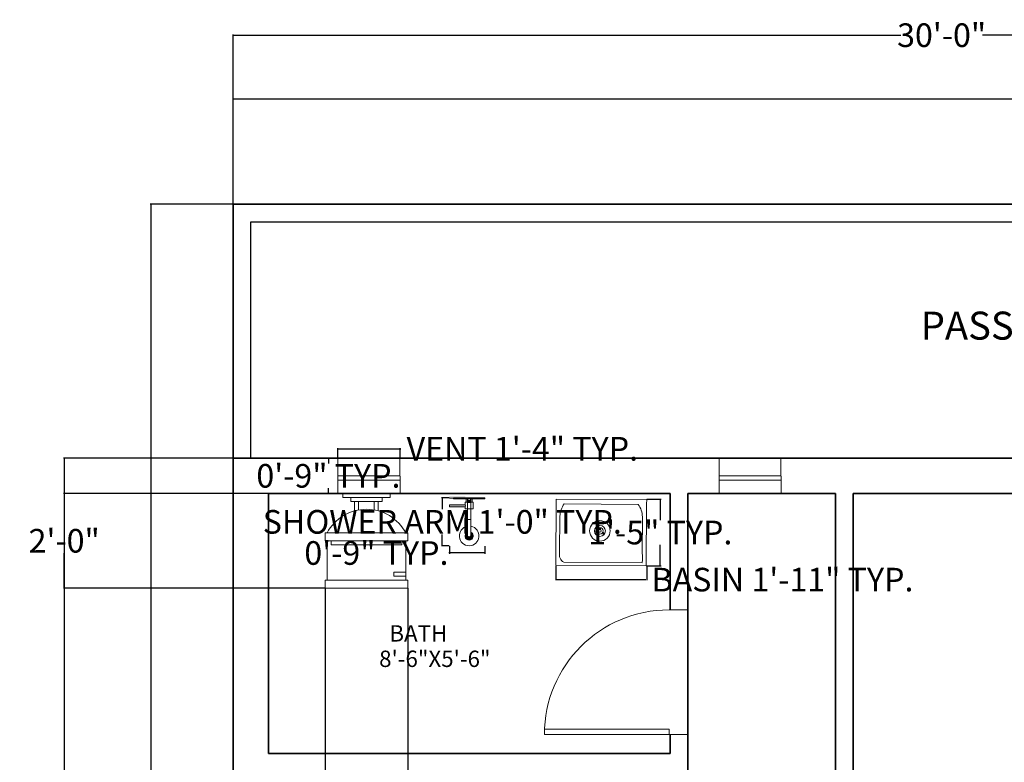
# Model space of a CAD drawing. Units: inches. Extents: x 79 to 8696167, y -3690578 to 147.
# Tile 5 of 10: x 79 to 329, y -42 to 147. Entities that reach past the tile are written whole.
import ezdxf

# ---------------------------------------------------------------- set-up
doc = ezdxf.new("R2010")
doc.units = ezdxf.units.IN
doc.header["$MEASUREMENT"] = 0
doc.layers.get('0').update_dxf_attribs({"color": 253})
for name, color, linetype, lineweight in [('A-ANNO-DIMS', 2, 'Continuous', 18), ('A-AREA-IDEN', 7, 'Continuous', 18), ('A-DOOR', 4, 'Continuous', 18), ('C-PROP', 7, 'Continuous', 35), ('C-SITE-WALL', 8, 'Continuous', 25), ('PLUMBING FIXTURES', 9, 'Continuous', 18), ('walls', 8, 'Continuous', 35), ('windows', 171, 'Continuous', 18)]:
    doc.layers.add(name, color=color, linetype=linetype, lineweight=lineweight)
doc.styles.get("Standard").update_dxf_attribs({"font": 'arial.ttf'})
doc.dimstyles.get("Standard").update_dxf_attribs({"dimtxt": 6, "dimasz": 0.18, "dimexe": 0.18, "dimexo": 0.0625, "dimgap": 0.09, "dimtad": 0, "dimtih": 1, "dimtoh": 1, "dimzin": 0, "dimdsep": 46, "dimlunit": 3, "dimtxsty": 'Standard', "dimcen": 0.09, "dimadec": 0, "dimazin": 0, "dimtfac": 1, "dimtofl": 0, "dimtmove": 0, "dimatfit": 3, "dimfxl": 1, "dimtolj": 1, "dimtzin": 0, "dimarcsym": 0})

# ---------------------------------------------------------------- blocks, each defined once
blk = doc.blocks.new('O.H SHOWER-PL')
at = {"layer": 'PLUMBING FIXTURES'}
for points in [[(-1.84, 0), (-1.84, -0.25), (1.84, -0.25), (1.84, 0)], [(0.46, -8.72), (0.46, -9.67, -0.422337), (-0.46, -9.67), (-0.46, -8.72, 4.325472)]]:
    blk.add_hatch(color=256, dxfattribs=at).paths.add_polyline_path(points)
for p, q in [((-1.84, 0), (-1.84, -0.25)), ((1.84, 0), (-1.84, 0)), ((1.84, 0), (1.84, -0.25)), ((1.84, -0.25), (-1.84, -0.25)), ((-0.46, -0.25), (-0.46, -9.67)), ((0.46, -0.25), (0.46, -9.67))]:
    blk.add_line(p, q, dxfattribs=at)
for centre, radius, start, end in [((0, -9.67), 2.5, 100.61, 79.39), ((0, -4.48), 1.03, 243.53, 296.47), ((0, -9.67), 1.05, 116.0349, 63.9652), ((0, -9.22), 0.643, 224.2078, 315.7922)]:
    blk.add_arc(centre, radius, start, end, dxfattribs=at)
blk = doc.blocks.new('DIVERTER-PL')
at = {"layer": 'PLUMBING FIXTURES'}
for points in [[(4, 0), (-4, 0), (-4, -0.25), (4, -0.25)], [(0.38, -1.14), (0.38, -0.7), (-0.37, -0.7), (-0.37, -1.14)], [(1, -1.75, 0.30818), (1, -2.25), (5, -2.25), (5, -1.75)]]:
    blk.add_hatch(color=256, dxfattribs=at).paths.add_polyline_path(points)
for p, q in [((-4, 0), (-4, -0.25)), ((-4, 0), (4, 0)), ((4, 0), (4, -0.25)), ((-4, -0.25), (4, -0.25)), ((-4, -0.25), (4, -0.25)), ((-1, -1.05), (-0.37, -1.05)), ((-1, -1.05), (-1, -2.75)), ((-0.75, -0.25), (-0.75, -1.05)), ((-0.37, -0.7), (0.38, -0.7)), ((-0.37, -0.7), (-0.37, -1.14)), ((-0.37, -1.14), (0.38, -1.14)), ((-0.32, -0.7), (-0.32, -0.25)), ((0.32, -0.7), (0.32, -0.25)), ((0.38, -0.7), (0.38, -1.14)), ((0.38, -1.05), (1, -1.05)), ((0.75, -0.25), (0.75, -1.05)), ((1, -1.05), (1, -1.75)), ((1, -2.25), (1, -2.75)), ((-1, -2.75), (1, -2.75))]:
    blk.add_line(p, q, dxfattribs=at)
at = {"layer": 'PLUMBING FIXTURES', "ltscale": 12}
for p, q in [((1, -1.75), (5, -1.75)), ((1, -2.25), (5, -2.25)), ((5, -2.25), (5, -1.75))]:
    blk.add_line(p, q, dxfattribs=at)
at = {"layer": 'PLUMBING FIXTURES'}
blk.add_arc((1.37, -2), 0.444, 145.7435, 214.2565, dxfattribs=at)
blk = doc.blocks.new('A$C7F153053')
at = {"layer": 'PLUMBING FIXTURES', "xscale": -1, "rotation": 270}
for name in ['DIVERTER-PL', 'O.H SHOWER-PL']:
    blk.add_blockref(name, (12.17, 4), dxfattribs=at)
blk = doc.blocks.new('*U10')
for p, q in [((-10, 22), (-10, 12)), ((-10, 21), (-7, 21)), ((-7, 21), (-7, 20)), ((10, 12), (10, 22)), ((-7, 20), (-10, 20)), ((9, 13), (-9, 13)), ((-9, 13), (-9, 12)), ((9, 12), (9, 13)), ((10.5, 12), (-10.5, 12)), ((-10.5, 10), (-10.5, 12)), ((10.5, 12), (10.5, 10)), ((10.5, 10), (-10.5, 10)), ((-3, 4.4065), (-3, 2)), ((-2, 2), (-2, 4.1658)), ((2, 4.1658), (2, 2)), ((3, 2), (3, 4.4065)), ((4, 2), (-4, 2)), ((-4, 2), (-4, 1)), ((4, 1), (4, 2))]:
    blk.add_line(p, q)
for points in [[(10.5, 22), (10.5, 24), (-10.5, 24), (-10.5, 22)], [(6, 0), (6, 1), (-6, 1), (-6, 0)]]:
    blk.add_lwpolyline(points, close=True)
blk.add_arc((0, 15.3333), 11.3333, 208.0725, 331.9275)
blk = doc.blocks.new('*U12')
for p, q in [((0, 0), (0, -6)), ((40, 0), (40, -6))]:
    blk.add_line(p, q)
blk.add_lwpolyline([(0, 0), (0, 40), (1.75, 40), (1.75, 0)], close=True)
blk.add_arc((0, 0), 40, 0, 90)
blk = doc.blocks.new('*D22')
at = {"layer": 'A-ANNO-DIMS', "color": 0, "lineweight": -2, "transparency": 16777216}
for p, q in [((133.44, 99.94), (133.44, 126.77)), ((133.62, 126.59), (338.26, 126.59)), ((553.26, 126.59), (348.62, 126.59)), ((553.44, 99.94), (553.44, 126.77))]:
    blk.add_line(p, q, dxfattribs=at)
at = {"layer": 'A-ANNO-DIMS', "color": 0, "lineweight": 100, "transparency": 16777216}
for points in [[(133.62, 126.62), (133.62, 126.56), (133.44, 126.59)], [(553.26, 126.62), (553.26, 126.56), (553.44, 126.59)]]:
    blk.add_solid(points, dxfattribs=at)
at = {"layer": 'Defpoints', "color": 0, "lineweight": 100, "transparency": 16777216}
for p in [(553.44, 126.59), (133.44, 99.88), (553.44, 99.88)]:
    blk.add_point(p, dxfattribs=at)
at = {"layer": 'A-ANNO-DIMS', "color": 0, "transparency": 16777216, "insert": (343.44, 126.59), "char_height": 6, "attachment_point": 5}
blk.add_mtext("\\A1;35'", dxfattribs=at)
blk = doc.blocks.new('*D23')
at = {"layer": 'A-ANNO-DIMS', "color": 0, "lineweight": -2, "transparency": 16777216}
for p, q in [((133.38, 99.88), (112.4, 99.88)), ((112.58, 99.7), (112.58, -286.97)), ((112.58, -679.94), (112.58, -293.28)), ((133.38, -680.12), (112.4, -680.12))]:
    blk.add_line(p, q, dxfattribs=at)
at = {"layer": 'A-ANNO-DIMS', "color": 0, "lineweight": 100, "transparency": 16777216}
for points in [[(112.55, 99.7), (112.61, 99.7), (112.58, 99.88)], [(112.55, -679.94), (112.61, -679.94), (112.58, -680.12)]]:
    blk.add_solid(points, dxfattribs=at)
at = {"layer": 'Defpoints', "color": 0, "lineweight": 100, "transparency": 16777216}
for p in [(112.58, 99.88), (133.44, 99.88), (133.44, -680.12)]:
    blk.add_point(p, dxfattribs=at)
at = {"layer": 'A-ANNO-DIMS', "color": 0, "transparency": 16777216, "insert": (112.58, -290.12), "char_height": 6, "attachment_point": 5}
blk.add_mtext("\\A1;65'", dxfattribs=at)
blk = doc.blocks.new('WIN-REAR-VENT')
for p, q in [((0, 0), (0, 9)), ((0, 9), (15.73, 9)), ((15.73, 9), (15.83, 0)), ((15.78, 4.5), (0, 4.5)), ((0, 0), (0, 3.42)), ((0, 3.42), (15.78, 3.42)), ((0.11, 0), (15.83, 0))]:
    blk.add_line(p, q)
blk = doc.blocks.new('BASIN-RECT-DRAIN')
for p, q in [((0, 0.15), (0.11, 17)), ((0.11, 17), (23.11, 16.85)), ((20.97, 15.65), (2.15, 15.77)), ((23.1, 15.71), (23, 0)), ((23.11, 16.85), (23.1, 15.71)), ((0.99, 3.35), (1.05, 12.64)), ((21.96, 3.21), (22.03, 12.5)), ((10.4, 8.91), (9.84, 8.81)), ((10.52, 8.7), (9.87, 8.58)), ((11.22, 9.73), (11.16, 9.24)), ((11.36, 9.22), (11.4, 9.7)), ((11.84, 8.39), (12.22, 7.95)), ((11.97, 8.6), (12.36, 8.13)), ((23, 0), (0, 0.15)), ((21.95, 0.84), (2.06, 0.97))]:
    blk.add_line(p, q)
for radius in [2.61, 1.39, 0.816, 0.338]:
    blk.add_circle((11.22, 8.91), radius)
for centre, radius, start, end in [((6.46, 12.5), 5.4, 142.7525, 178.5493), ((16.62, 12.43), 5.4, 0.6949, 36.4918), ((3, 2.82), 2.08, 165.2338, 242.9258), ((12.7, 2.09), 9.33, 352.3124, 6.9318)]:
    blk.add_arc(centre, radius, start, end)
blk = doc.blocks.new('SHOWER-HEAD-DETAIL')
for points in [[(4, 12.56, -0.30818), (4, 12.06), (0, 12.06), (0, 12.56)], [(4, 12.56, -0.30818), (4, 12.06), (0, 12.06), (0, 12.56)], [(4, 12.56, -0.30818), (4, 12.06), (0, 12.06), (0, 12.56)], [(4, 12.56, -0.30818), (4, 12.06), (0, 12.06), (0, 12.56)], [(4, 12.56, -0.30818), (4, 12.06), (0, 12.06), (0, 12.56)], [(4, 12.56, -0.30818), (4, 12.06), (0, 12.06), (0, 12.56)], [(4, 12.56, -0.30818), (4, 12.06), (0, 12.06), (0, 12.56)], [(4, 12.56, -0.30818), (4, 12.06), (0, 12.06), (0, 12.56)], [(4, 12.56, -0.30818), (4, 12.06), (0, 12.06), (0, 12.56)], [(4, 12.56, -0.30818), (4, 12.06), (0, 12.06), (0, 12.56)], [(4, 12.56, -0.30818), (4, 12.06), (0, 12.06), (0, 12.56)], [(4, 12.56, -0.30818), (4, 12.06), (0, 12.06), (0, 12.56)], [(4, 12.56, -0.30818), (4, 12.06), (0, 12.06), (0, 12.56)], [(4, 12.56, -0.30818), (4, 12.06), (0, 12.06), (0, 12.56)], [(4, 12.56, -0.30818), (4, 12.06), (0, 12.06), (0, 12.56)], [(4, 12.56, -0.30818), (4, 12.06), (0, 12.06), (0, 12.56)], [(4, 12.56, -0.30818), (4, 12.06), (0, 12.06), (0, 12.56)], [(4, 12.56, -0.30818), (4, 12.06), (0, 12.06), (0, 12.56)], [(4, 12.56, -0.30818), (4, 12.06), (0, 12.06), (0, 12.56)], [(4, 12.56, -0.30818), (4, 12.06), (0, 12.06), (0, 12.56)], [(4, 12.56, -0.30818), (4, 12.06), (0, 12.06), (0, 12.56)], [(4, 12.56, -0.30818), (4, 12.06), (0, 12.06), (0, 12.56)], [(4, 12.56, -0.30818), (4, 12.06), (0, 12.06), (0, 12.56)], [(4, 12.56, -0.30818), (4, 12.06), (0, 12.06), (0, 12.56)], [(4, 12.56, -0.30818), (4, 12.06), (0, 12.06), (0, 12.56)], [(4, 12.56, -0.30818), (4, 12.06), (0, 12.06), (0, 12.56)], [(4, 12.56, -0.30818), (4, 12.06), (0, 12.06), (0, 12.56)], [(4, 12.56, -0.30818), (4, 12.06), (0, 12.06), (0, 12.56)], [(4, 12.56, -0.30818), (4, 12.06), (0, 12.06), (0, 12.56)], [(4, 12.56, -0.30818), (4, 12.06), (0, 12.06), (0, 12.56)], [(4, 12.56, -0.30818), (4, 12.06), (0, 12.06), (0, 12.56)], [(4, 12.56, -0.30818), (4, 12.06), (0, 12.06), (0, 12.56)], [(4, 12.56, -0.30818), (4, 12.06), (0, 12.06), (0, 12.56)], [(4, 12.56, -0.30818), (4, 12.06), (0, 12.06), (0, 12.56)], [(4, 12.56, -0.30818), (4, 12.06), (0, 12.06), (0, 12.56)], [(4, 12.56, -0.30818), (4, 12.06), (0, 12.06), (0, 12.56)], [(4.54, 3.44), (4.54, 2.5, 0.422337), (5.46, 2.5), (5.46, 3.44, -4.325472)], [(4.54, 3.44), (4.54, 2.5, 0.422337), (5.46, 2.5), (5.46, 3.44, -4.325472)], [(4.54, 3.44), (4.54, 2.5, 0.422337), (5.46, 2.5), (5.46, 3.44, -4.325472)], [(4.54, 3.44), (4.54, 2.5, 0.422337), (5.46, 2.5), (5.46, 3.44, -4.325472)], [(4.54, 3.44), (4.54, 2.5, 0.422337), (5.46, 2.5), (5.46, 3.44, -4.325472)], [(4.54, 3.44), (4.54, 2.5, 0.422337), (5.46, 2.5), (5.46, 3.44, -4.325472)], [(4.54, 3.44), (4.54, 2.5, 0.422337), (5.46, 2.5), (5.46, 3.44, -4.325472)], [(4.54, 3.44), (4.54, 2.5, 0.422337), (5.46, 2.5), (5.46, 3.44, -4.325472)], [(4.54, 3.44), (4.54, 2.5, 0.422337), (5.46, 2.5), (5.46, 3.44, -4.325472)], [(4.54, 3.44), (4.54, 2.5, 0.422337), (5.46, 2.5), (5.46, 3.44, -4.325472)], [(4.54, 3.44), (4.54, 2.5, 0.422337), (5.46, 2.5), (5.46, 3.44, -4.325472)], [(4.54, 3.44), (4.54, 2.5, 0.422337), (5.46, 2.5), (5.46, 3.44, -4.325472)], [(4.54, 3.44), (4.54, 2.5, 0.422337), (5.46, 2.5), (5.46, 3.44, -4.325472)], [(4.54, 3.44), (4.54, 2.5, 0.422337), (5.46, 2.5), (5.46, 3.44, -4.325472)], [(4.54, 3.44), (4.54, 2.5, 0.422337), (5.46, 2.5), (5.46, 3.44, -4.325472)], [(4.54, 3.44), (4.54, 2.5, 0.422337), (5.46, 2.5), (5.46, 3.44, -4.325472)], [(4.54, 3.44), (4.54, 2.5, 0.422337), (5.46, 2.5), (5.46, 3.44, -4.325472)], [(4.54, 3.44), (4.54, 2.5, 0.422337), (5.46, 2.5), (5.46, 3.44, -4.325472)], [(4.54, 3.44), (4.54, 2.5, 0.422337), (5.46, 2.5), (5.46, 3.44, -4.325472)], [(4.54, 3.44), (4.54, 2.5, 0.422337), (5.46, 2.5), (5.46, 3.44, -4.325472)], [(4.54, 3.44), (4.54, 2.5, 0.422337), (5.46, 2.5), (5.46, 3.44, -4.325472)], [(4.54, 3.44), (4.54, 2.5, 0.422337), (5.46, 2.5), (5.46, 3.44, -4.325472)], [(4.54, 3.44), (4.54, 2.5, 0.422337), (5.46, 2.5), (5.46, 3.44, -4.325472)], [(4.54, 3.44), (4.54, 2.5, 0.422337), (5.46, 2.5), (5.46, 3.44, -4.325472)], [(4.54, 3.44), (4.54, 2.5, 0.422337), (5.46, 2.5), (5.46, 3.44, -4.325472)], [(4.54, 3.44), (4.54, 2.5, 0.422337), (5.46, 2.5), (5.46, 3.44, -4.325472)], [(4.54, 3.44), (4.54, 2.5, 0.422337), (5.46, 2.5), (5.46, 3.44, -4.325472)], [(4.54, 3.44), (4.54, 2.5, 0.422337), (5.46, 2.5), (5.46, 3.44, -4.325472)], [(4.54, 3.44), (4.54, 2.5, 0.422337), (5.46, 2.5), (5.46, 3.44, -4.325472)], [(4.54, 3.44), (4.54, 2.5, 0.422337), (5.46, 2.5), (5.46, 3.44, -4.325472)], [(4.54, 3.44), (4.54, 2.5, 0.422337), (5.46, 2.5), (5.46, 3.44, -4.325472)], [(4.54, 3.44), (4.54, 2.5, 0.422337), (5.46, 2.5), (5.46, 3.44, -4.325472)], [(4.54, 3.44), (4.54, 2.5, 0.422337), (5.46, 2.5), (5.46, 3.44, -4.325472)], [(4.54, 3.44), (4.54, 2.5, 0.422337), (5.46, 2.5), (5.46, 3.44, -4.325472)], [(4.54, 3.44), (4.54, 2.5, 0.422337), (5.46, 2.5), (5.46, 3.44, -4.325472)], [(4.54, 3.44), (4.54, 2.5, 0.422337), (5.46, 2.5), (5.46, 3.44, -4.325472)], [(4.54, 3.44), (4.54, 2.5, 0.422337), (5.46, 2.5), (5.46, 3.44, -4.325472)], [(4.54, 3.44), (4.54, 2.5, 0.422337), (5.46, 2.5), (5.46, 3.44, -4.325472)]]:
    blk.add_hatch(color=256).paths.add_polyline_path(points)
at = {"ltscale": 12}
blk.add_line((4, 12.06), (0, 12.06), dxfattribs=at)
blk.add_line((4, 12.06), (0, 12.06), dxfattribs=at)
blk.add_line((4, 12.06), (0, 12.06), dxfattribs=at)
blk.add_line((4, 12.06), (0, 12.06), dxfattribs=at)
blk.add_line((4, 12.06), (0, 12.06), dxfattribs=at)
blk.add_line((4, 12.06), (0, 12.06), dxfattribs=at)
blk.add_line((4, 12.06), (0, 12.06), dxfattribs=at)
blk.add_line((4, 12.06), (0, 12.06), dxfattribs=at)
blk.add_line((4, 12.06), (0, 12.06), dxfattribs=at)
blk.add_line((4, 12.06), (0, 12.06), dxfattribs=at)
blk.add_line((4, 12.06), (0, 12.06), dxfattribs=at)
blk.add_line((4, 12.06), (0, 12.06), dxfattribs=at)
blk.add_line((4, 12.06), (0, 12.06), dxfattribs=at)
blk.add_line((4, 12.06), (0, 12.06), dxfattribs=at)
blk.add_line((4, 12.06), (0, 12.06), dxfattribs=at)
blk.add_line((4, 12.06), (0, 12.06), dxfattribs=at)
blk.add_line((4, 12.06), (0, 12.06), dxfattribs=at)
blk.add_line((4, 12.06), (0, 12.06), dxfattribs=at)
blk.add_line((4, 12.06), (0, 12.06), dxfattribs=at)
blk.add_line((4, 12.06), (0, 12.06), dxfattribs=at)
blk.add_line((4, 12.06), (0, 12.06), dxfattribs=at)
blk.add_line((4, 12.06), (0, 12.06), dxfattribs=at)
blk.add_line((4, 12.06), (0, 12.06), dxfattribs=at)
blk.add_line((4, 12.06), (0, 12.06), dxfattribs=at)
blk.add_line((4, 12.06), (0, 12.06), dxfattribs=at)
blk.add_line((4, 12.06), (0, 12.06), dxfattribs=at)
blk.add_line((4, 12.06), (0, 12.06), dxfattribs=at)
blk.add_line((4, 12.06), (0, 12.06), dxfattribs=at)
blk.add_line((4, 12.06), (0, 12.06), dxfattribs=at)
blk.add_line((4, 12.06), (0, 12.06), dxfattribs=at)
blk.add_line((4, 12.06), (0, 12.06), dxfattribs=at)
blk.add_line((4, 12.06), (0, 12.06), dxfattribs=at)
blk.add_line((4, 12.06), (0, 12.06), dxfattribs=at)
blk.add_line((4, 12.06), (0, 12.06), dxfattribs=at)
blk.add_line((4, 12.06), (0, 12.06), dxfattribs=at)
blk.add_line((4, 12.06), (0, 12.06), dxfattribs=at)
blk.add_line((4, 12.06), (0, 12.06), dxfattribs=at)
blk.add_line((4, 12.06), (0, 12.06), dxfattribs=at)
for p, q in [((4.54, 11.92), (4.54, 2.5)), ((4.54, 11.92), (4.54, 2.5)), ((4.54, 11.92), (4.54, 2.5)), ((4.54, 11.92), (4.54, 2.5)), ((4.54, 11.92), (4.54, 2.5)), ((4.54, 11.92), (4.54, 2.5)), ((4.54, 11.92), (4.54, 2.5)), ((4.54, 11.92), (4.54, 2.5)), ((4.54, 11.92), (4.54, 2.5)), ((4.54, 11.92), (4.54, 2.5)), ((4.54, 11.92), (4.54, 2.5)), ((4.54, 11.92), (4.54, 2.5)), ((4.54, 11.92), (4.54, 2.5)), ((4.54, 11.92), (4.54, 2.5)), ((4.54, 11.92), (4.54, 2.5)), ((4.54, 11.92), (4.54, 2.5)), ((4.54, 11.92), (4.54, 2.5)), ((4.54, 11.92), (4.54, 2.5)), ((4.54, 11.92), (4.54, 2.5)), ((4.54, 11.92), (4.54, 2.5)), ((4.54, 11.92), (4.54, 2.5)), ((4.54, 11.92), (4.54, 2.5)), ((4.54, 11.92), (4.54, 2.5)), ((4.54, 11.92), (4.54, 2.5)), ((4.54, 11.92), (4.54, 2.5)), ((4.54, 11.92), (4.54, 2.5)), ((4.54, 11.92), (4.54, 2.5)), ((4.54, 11.92), (4.54, 2.5)), ((4.54, 11.92), (4.54, 2.5)), ((4.54, 11.92), (4.54, 2.5)), ((4.54, 11.92), (4.54, 2.5)), ((4.54, 11.92), (4.54, 2.5)), ((4.54, 11.92), (4.54, 2.5)), ((4.54, 11.92), (4.54, 2.5)), ((4.54, 11.92), (4.54, 2.5)), ((4.54, 11.92), (4.54, 2.5)), ((4.54, 11.92), (4.54, 2.5)), ((4.54, 11.92), (4.54, 2.5)), ((5.46, 11.92), (5.46, 2.5)), ((5.46, 11.92), (5.46, 2.5)), ((5.46, 11.92), (5.46, 2.5)), ((5.46, 11.92), (5.46, 2.5)), ((5.46, 11.92), (5.46, 2.5)), ((5.46, 11.92), (5.46, 2.5)), ((5.46, 11.92), (5.46, 2.5)), ((5.46, 11.92), (5.46, 2.5)), ((5.46, 11.92), (5.46, 2.5)), ((5.46, 11.92), (5.46, 2.5)), ((5.46, 11.92), (5.46, 2.5)), ((5.46, 11.92), (5.46, 2.5)), ((5.46, 11.92), (5.46, 2.5)), ((5.46, 11.92), (5.46, 2.5)), ((5.46, 11.92), (5.46, 2.5)), ((5.46, 11.92), (5.46, 2.5)), ((5.46, 11.92), (5.46, 2.5)), ((5.46, 11.92), (5.46, 2.5)), ((5.46, 11.92), (5.46, 2.5)), ((5.46, 11.92), (5.46, 2.5)), ((5.46, 11.92), (5.46, 2.5)), ((5.46, 11.92), (5.46, 2.5)), ((5.46, 11.92), (5.46, 2.5)), ((5.46, 11.92), (5.46, 2.5)), ((5.46, 11.92), (5.46, 2.5)), ((5.46, 11.92), (5.46, 2.5)), ((5.46, 11.92), (5.46, 2.5)), ((5.46, 11.92), (5.46, 2.5)), ((5.46, 11.92), (5.46, 2.5)), ((5.46, 11.92), (5.46, 2.5)), ((5.46, 11.92), (5.46, 2.5)), ((5.46, 11.92), (5.46, 2.5)), ((5.46, 11.92), (5.46, 2.5)), ((5.46, 11.92), (5.46, 2.5)), ((5.46, 11.92), (5.46, 2.5)), ((5.46, 11.92), (5.46, 2.5)), ((5.46, 11.92), (5.46, 2.5)), ((5.46, 11.92), (5.46, 2.5))]:
    blk.add_line(p, q)
for centre, radius, start, end in [((5, 7.69), 1.03, 243.53, 296.47), ((5, 7.69), 1.03, 243.53, 296.47), ((5, 7.69), 1.03, 243.53, 296.47), ((5, 7.69), 1.03, 243.53, 296.47), ((5, 7.69), 1.03, 243.53, 296.47), ((5, 7.69), 1.03, 243.53, 296.47), ((5, 7.69), 1.03, 243.53, 296.47), ((5, 7.69), 1.03, 243.53, 296.47), ((5, 7.69), 1.03, 243.53, 296.47), ((5, 7.69), 1.03, 243.53, 296.47), ((5, 7.69), 1.03, 243.53, 296.47), ((5, 7.69), 1.03, 243.53, 296.47), ((5, 7.69), 1.03, 243.53, 296.47), ((5, 7.69), 1.03, 243.53, 296.47), ((5, 7.69), 1.03, 243.53, 296.47), ((5, 7.69), 1.03, 243.53, 296.47), ((5, 7.69), 1.03, 243.53, 296.47), ((5, 7.69), 1.03, 243.53, 296.47), ((5, 7.69), 1.03, 243.53, 296.47), ((5, 7.69), 1.03, 243.53, 296.47), ((5, 7.69), 1.03, 243.53, 296.47), ((5, 7.69), 1.03, 243.53, 296.47), ((5, 7.69), 1.03, 243.53, 296.47), ((5, 7.69), 1.03, 243.53, 296.47), ((5, 7.69), 1.03, 243.53, 296.47), ((5, 7.69), 1.03, 243.53, 296.47), ((5, 7.69), 1.03, 243.53, 296.47), ((5, 7.69), 1.03, 243.53, 296.47), ((5, 7.69), 1.03, 243.53, 296.47), ((5, 7.69), 1.03, 243.53, 296.47), ((5, 7.69), 1.03, 243.53, 296.47), ((5, 7.69), 1.03, 243.53, 296.47), ((5, 7.69), 1.03, 243.53, 296.47), ((5, 7.69), 1.03, 243.53, 296.47), ((5, 7.69), 1.03, 243.53, 296.47), ((5, 7.69), 1.03, 243.53, 296.47), ((5, 7.69), 1.03, 243.53, 296.47), ((5, 7.69), 1.03, 243.53, 296.47), ((5, 2.5), 2.5, 100.61, 79.39), ((5, 2.5), 2.5, 100.61, 79.39), ((5, 2.5), 2.5, 100.61, 79.39), ((5, 2.5), 2.5, 100.61, 79.39), ((5, 2.5), 2.5, 100.61, 79.39), ((5, 2.5), 2.5, 100.61, 79.39), ((5, 2.5), 2.5, 100.61, 79.39), ((5, 2.5), 2.5, 100.61, 79.39), ((5, 2.5), 2.5, 100.61, 79.39), ((5, 2.5), 2.5, 100.61, 79.39), ((5, 2.5), 2.5, 100.61, 79.39), ((5, 2.5), 2.5, 100.61, 79.39), ((5, 2.5), 2.5, 100.61, 79.39), ((5, 2.5), 2.5, 100.61, 79.39), ((5, 2.5), 2.5, 100.61, 79.39), ((5, 2.5), 2.5, 100.61, 79.39), ((5, 2.5), 2.5, 100.61, 79.39), ((5, 2.5), 2.5, 100.61, 79.39), ((5, 2.5), 2.5, 100.61, 79.39), ((5, 2.5), 2.5, 100.61, 79.39), ((5, 2.5), 2.5, 100.61, 79.39), ((5, 2.5), 2.5, 100.61, 79.39), ((5, 2.5), 2.5, 100.61, 79.39), ((5, 2.5), 2.5, 100.61, 79.39), ((5, 2.5), 2.5, 100.61, 79.39), ((5, 2.5), 2.5, 100.61, 79.39), ((5, 2.5), 2.5, 100.61, 79.39), ((5, 2.5), 2.5, 100.61, 79.39), ((5, 2.5), 2.5, 100.61, 79.39), ((5, 2.5), 2.5, 100.61, 79.39), ((5, 2.5), 2.5, 100.61, 79.39), ((5, 2.5), 2.5, 100.61, 79.39), ((5, 2.5), 2.5, 100.61, 79.39), ((5, 2.5), 2.5, 100.61, 79.39), ((5, 2.5), 2.5, 100.61, 79.39), ((5, 2.5), 2.5, 100.61, 79.39), ((5, 2.5), 2.5, 100.61, 79.39), ((5, 2.5), 2.5, 100.61, 79.39), ((5, 2.5), 1.05, 116.0348, 63.9651), ((5, 2.5), 1.05, 116.0348, 63.9651), ((5, 2.5), 1.05, 116.0348, 63.9651), ((5, 2.5), 1.05, 116.0348, 63.9651), ((5, 2.5), 1.05, 116.0348, 63.9651), ((5, 2.5), 1.05, 116.0348, 63.9651), ((5, 2.5), 1.05, 116.0348, 63.9651), ((5, 2.5), 1.05, 116.0348, 63.9651), ((5, 2.5), 1.05, 116.0348, 63.9651), ((5, 2.5), 1.05, 116.0348, 63.9651), ((5, 2.5), 1.05, 116.0348, 63.9651), ((5, 2.5), 1.05, 116.0348, 63.9651), ((5, 2.5), 1.05, 116.0348, 63.9651), ((5, 2.5), 1.05, 116.0348, 63.9651), ((5, 2.5), 1.05, 116.0348, 63.9651), ((5, 2.5), 1.05, 116.0348, 63.9651), ((5, 2.5), 1.05, 116.0348, 63.9651), ((5, 2.5), 1.05, 116.0348, 63.9651), ((5, 2.5), 1.05, 116.0348, 63.9651), ((5, 2.5), 1.05, 116.0348, 63.9651), ((5, 2.5), 1.05, 116.0348, 63.9651), ((5, 2.5), 1.05, 116.0348, 63.9651), ((5, 2.5), 1.05, 116.0348, 63.9651), ((5, 2.5), 1.05, 116.0348, 63.9651), ((5, 2.5), 1.05, 116.0348, 63.9651), ((5, 2.5), 1.05, 116.0348, 63.9651), ((5, 2.5), 1.05, 116.0348, 63.9651), ((5, 2.5), 1.05, 116.0348, 63.9651), ((5, 2.5), 1.05, 116.0348, 63.9651), ((5, 2.5), 1.05, 116.0348, 63.9651), ((5, 2.5), 1.05, 116.0348, 63.9651), ((5, 2.5), 1.05, 116.0348, 63.9651), ((5, 2.5), 1.05, 116.0348, 63.9651), ((5, 2.5), 1.05, 116.0348, 63.9651), ((5, 2.5), 1.05, 116.0348, 63.9651), ((5, 2.5), 1.05, 116.0348, 63.9651), ((5, 2.5), 1.05, 116.0348, 63.9651), ((5, 2.5), 1.05, 116.0348, 63.9651), ((5, 2.95), 0.643, 224.2078, 315.7922), ((5, 2.95), 0.643, 224.2078, 315.7922), ((5, 2.95), 0.643, 224.2078, 315.7922), ((5, 2.95), 0.643, 224.2078, 315.7922), ((5, 2.95), 0.643, 224.2078, 315.7922), ((5, 2.95), 0.643, 224.2078, 315.7922), ((5, 2.95), 0.643, 224.2078, 315.7922), ((5, 2.95), 0.643, 224.2078, 315.7922), ((5, 2.95), 0.643, 224.2078, 315.7922), ((5, 2.95), 0.643, 224.2078, 315.7922), ((5, 2.95), 0.643, 224.2078, 315.7922), ((5, 2.95), 0.643, 224.2078, 315.7922), ((5, 2.95), 0.643, 224.2078, 315.7922), ((5, 2.95), 0.643, 224.2078, 315.7922), ((5, 2.95), 0.643, 224.2078, 315.7922), ((5, 2.95), 0.643, 224.2078, 315.7922), ((5, 2.95), 0.643, 224.2078, 315.7922), ((5, 2.95), 0.643, 224.2078, 315.7922), ((5, 2.95), 0.643, 224.2078, 315.7922), ((5, 2.95), 0.643, 224.2078, 315.7922), ((5, 2.95), 0.643, 224.2078, 315.7922), ((5, 2.95), 0.643, 224.2078, 315.7922), ((5, 2.95), 0.643, 224.2078, 315.7922), ((5, 2.95), 0.643, 224.2078, 315.7922), ((5, 2.95), 0.643, 224.2078, 315.7922), ((5, 2.95), 0.643, 224.2078, 315.7922), ((5, 2.95), 0.643, 224.2078, 315.7922), ((5, 2.95), 0.643, 224.2078, 315.7922), ((5, 2.95), 0.643, 224.2078, 315.7922), ((5, 2.95), 0.643, 224.2078, 315.7922), ((5, 2.95), 0.643, 224.2078, 315.7922), ((5, 2.95), 0.643, 224.2078, 315.7922), ((5, 2.95), 0.643, 224.2078, 315.7922), ((5, 2.95), 0.643, 224.2078, 315.7922), ((5, 2.95), 0.643, 224.2078, 315.7922), ((5, 2.95), 0.643, 224.2078, 315.7922), ((5, 2.95), 0.643, 224.2078, 315.7922), ((5, 2.95), 0.643, 224.2078, 315.7922)]:
    blk.add_arc(centre, radius, start, end)
blk = doc.blocks.new('*D31')
at = {"layer": 'A-ANNO-DIMS', "color": 0, "lineweight": -2, "transparency": 16777216}
for p, q in [((160.03, 35.44), (160.03, 37.93)), ((160.21, 37.75), (175.69, 37.75)), ((175.87, 35.44), (175.87, 37.93)), ((175.87, 37.75), (176.05, 37.75))]:
    blk.add_line(p, q, dxfattribs=at)
at = {"layer": 'A-ANNO-DIMS', "color": 0, "lineweight": 100, "transparency": 16777216}
for points in [[(160.21, 37.78), (160.21, 37.72), (160.03, 37.75)], [(175.69, 37.78), (175.69, 37.72), (175.87, 37.75)]]:
    blk.add_solid(points, dxfattribs=at)
at = {"layer": 'Defpoints', "color": 0, "lineweight": 100, "transparency": 16777216}
for p in [(175.87, 37.75), (160.03, 35.38), (175.87, 35.38)]:
    blk.add_point(p, dxfattribs=at)
at = {"layer": 'A-ANNO-DIMS', "color": 0, "transparency": 16777216, "insert": (206.92, 37.75), "char_height": 6, "attachment_point": 5}
blk.add_mtext('\\A1;VENT 1\'-4" TYP.', dxfattribs=at)
blk = doc.blocks.new('*D32')
at = {"layer": 'A-ANNO-DIMS', "color": 0, "lineweight": -2, "transparency": 16777216}
for p, q in [((159.97, 35.38), (157.48, 35.38)), ((157.66, 35.2), (157.66, 34.03)), ((157.66, 26.56), (157.66, 27.72)), ((159.97, 26.38), (157.48, 26.38))]:
    blk.add_line(p, q, dxfattribs=at)
at = {"layer": 'A-ANNO-DIMS', "color": 0, "lineweight": 100, "transparency": 16777216}
for points in [[(157.63, 35.2), (157.69, 35.2), (157.66, 35.38)], [(157.63, 26.56), (157.69, 26.56), (157.66, 26.38)]]:
    blk.add_solid(points, dxfattribs=at)
at = {"layer": 'Defpoints', "color": 0, "lineweight": 100, "transparency": 16777216}
for p in [(157.66, 35.38), (160.03, 35.38), (160.03, 26.38)]:
    blk.add_point(p, dxfattribs=at)
at = {"layer": 'A-ANNO-DIMS', "color": 0, "transparency": 16777216, "insert": (157.66, 30.88), "char_height": 6, "attachment_point": 5}
blk.add_mtext('\\A1;0\'-9" TYP.', dxfattribs=at)
blk = doc.blocks.new('*D43')
at = {"layer": 'A-ANNO-DIMS', "color": 0, "lineweight": -2, "transparency": 16777216}
for p, q in [((188.35, 25.27), (186.4, 25.27)), ((186.58, 25.09), (186.58, 22.38)), ((186.58, 13.28), (186.58, 15.99)), ((188.35, 13.1), (186.4, 13.1))]:
    blk.add_line(p, q, dxfattribs=at)
at = {"layer": 'A-ANNO-DIMS', "color": 0, "lineweight": 100, "transparency": 16777216}
for points in [[(186.55, 25.09), (186.61, 25.09), (186.58, 25.27)], [(186.55, 13.28), (186.61, 13.28), (186.58, 13.1)]]:
    blk.add_solid(points, dxfattribs=at)
at = {"layer": 'Defpoints', "color": 0, "lineweight": 100, "transparency": 16777216}
for p in [(186.58, 25.27), (188.41, 25.27), (188.41, 13.1)]:
    blk.add_point(p, dxfattribs=at)
at = {"layer": 'A-ANNO-DIMS', "color": 0, "transparency": 16777216, "insert": (186.58, 19.19), "char_height": 6, "attachment_point": 5}
blk.add_mtext('\\A1;SHOWER ARM 1\'-0" TYP.', dxfattribs=at)
blk = doc.blocks.new('*D44')
at = {"layer": 'A-ANNO-DIMS', "color": 0, "lineweight": -2, "transparency": 16777216}
for p, q in [((188.41, 13.04), (188.41, 11.1)), ((197.41, 13.04), (197.41, 11.1)), ((188.41, 11.28), (188.23, 11.28)), ((197.23, 11.28), (188.59, 11.28))]:
    blk.add_line(p, q, dxfattribs=at)
at = {"layer": 'A-ANNO-DIMS', "color": 0, "lineweight": 100, "transparency": 16777216}
for points in [[(188.59, 11.31), (188.59, 11.25), (188.41, 11.28)], [(197.23, 11.31), (197.23, 11.25), (197.41, 11.28)]]:
    blk.add_solid(points, dxfattribs=at)
at = {"layer": 'Defpoints', "color": 0, "lineweight": 100, "transparency": 16777216}
for p in [(188.41, 13.1), (197.41, 13.1), (188.41, 11.28)]:
    blk.add_point(p, dxfattribs=at)
at = {"layer": 'A-ANNO-DIMS', "color": 0, "transparency": 16777216, "insert": (169.85, 11.28), "char_height": 6, "attachment_point": 5}
blk.add_mtext('\\A1;0\'-9" TYP.', dxfattribs=at)
blk = doc.blocks.new('*D47')
at = {"layer": 'A-ANNO-DIMS', "color": 0, "lineweight": -2, "transparency": 16777216}
for p, q in [((215.4, 7.92), (215.4, 4.34)), ((238.51, 7.92), (238.51, 4.34)), ((215.58, 4.52), (238.33, 4.52)), ((238.51, 4.52), (238.69, 4.52))]:
    blk.add_line(p, q, dxfattribs=at)
at = {"layer": 'A-ANNO-DIMS', "color": 0, "lineweight": 100, "transparency": 16777216}
for points in [[(215.58, 4.55), (215.58, 4.49), (215.4, 4.52)], [(238.33, 4.55), (238.33, 4.49), (238.51, 4.52)]]:
    blk.add_solid(points, dxfattribs=at)
at = {"layer": 'Defpoints', "color": 0, "lineweight": 100, "transparency": 16777216}
for p in [(215.4, 7.98), (238.51, 7.98), (238.51, 4.52)]:
    blk.add_point(p, dxfattribs=at)
at = {"layer": 'A-ANNO-DIMS', "color": 0, "transparency": 16777216, "insert": (273, 4.52), "char_height": 6, "attachment_point": 5}
blk.add_mtext('\\A1;BASIN 1\'-11" TYP.', dxfattribs=at)
blk = doc.blocks.new('*D48')
at = {"layer": 'A-ANNO-DIMS', "color": 0, "lineweight": -2, "transparency": 16777216}
for p, q in [((238.57, 24.98), (242.15, 24.98)), ((241.97, 24.8), (241.97, 19.64)), ((241.97, 8.16), (241.97, 13.33)), ((238.57, 7.98), (242.15, 7.98))]:
    blk.add_line(p, q, dxfattribs=at)
at = {"layer": 'A-ANNO-DIMS', "color": 0, "lineweight": 100, "transparency": 16777216}
for points in [[(241.94, 24.8), (242, 24.8), (241.97, 24.98)], [(241.94, 8.16), (242, 8.16), (241.97, 7.98)]]:
    blk.add_solid(points, dxfattribs=at)
at = {"layer": 'Defpoints', "color": 0, "lineweight": 100, "transparency": 16777216}
for p in [(238.51, 24.98), (241.97, 24.98), (238.51, 7.98)]:
    blk.add_point(p, dxfattribs=at)
at = {"layer": 'A-ANNO-DIMS', "color": 0, "transparency": 16777216, "insert": (241.97, 16.48), "char_height": 6, "attachment_point": 5}
blk.add_mtext('\\A1;1\'-5" TYP.', dxfattribs=at)
blk = doc.blocks.new('*D55')
at = {"layer": 'A-ANNO-DIMS', "color": 0, "lineweight": -2, "transparency": 16777216}
for p, q in [((133.44, 35.44), (133.44, 142.96)), ((133.62, 142.78), (303.05, 142.78)), ((493.26, 142.78), (323.83, 142.78)), ((493.44, 35.44), (493.44, 142.96))]:
    blk.add_line(p, q, dxfattribs=at)
at = {"layer": 'A-ANNO-DIMS', "color": 0, "lineweight": 100, "transparency": 16777216}
for points in [[(133.62, 142.81), (133.62, 142.75), (133.44, 142.78)], [(493.26, 142.81), (493.26, 142.75), (493.44, 142.78)]]:
    blk.add_solid(points, dxfattribs=at)
at = {"layer": 'Defpoints', "color": 0, "lineweight": 100, "transparency": 16777216}
for p in [(493.44, 142.78), (133.44, 35.38), (493.44, 35.38)]:
    blk.add_point(p, dxfattribs=at)
at = {"layer": 'A-ANNO-DIMS', "color": 0, "transparency": 16777216, "insert": (313.44, 142.78), "char_height": 6, "attachment_point": 5}
blk.add_mtext('\\A1;30\'-0"', dxfattribs=at)
blk = doc.blocks.new('*D56')
at = {"layer": 'A-ANNO-DIMS', "color": 0, "lineweight": -2, "transparency": 16777216}
for p, q in [((133.38, 35.38), (90.36, 35.38)), ((90.54, 35.2), (90.54, -253.97)), ((90.54, -549.44), (90.54, -260.28)), ((133.38, -549.62), (90.36, -549.62))]:
    blk.add_line(p, q, dxfattribs=at)
at = {"layer": 'A-ANNO-DIMS', "color": 0, "lineweight": 100, "transparency": 16777216}
for points in [[(90.51, 35.2), (90.57, 35.2), (90.54, 35.38)], [(90.51, -549.44), (90.57, -549.44), (90.54, -549.62)]]:
    blk.add_solid(points, dxfattribs=at)
at = {"layer": 'Defpoints', "color": 0, "lineweight": 100, "transparency": 16777216}
for p in [(90.54, 35.38), (133.44, 35.38), (133.44, -549.62)]:
    blk.add_point(p, dxfattribs=at)
at = {"layer": 'A-ANNO-DIMS', "color": 0, "transparency": 16777216, "insert": (90.54, -257.12), "char_height": 6, "attachment_point": 5}
blk.add_mtext('\\A1;48\'-9"', dxfattribs=at)
blk = doc.blocks.new('*D59')
at = {"layer": 'A-ANNO-DIMS', "color": 0, "lineweight": -2, "transparency": 16777216}
for p, q in [((156.82, 2.31), (156.82, -723.2)), ((177.82, 2.31), (177.82, -723.2)), ((157, -723.02), (159.53, -723.02)), ((177.64, -723.02), (175.1, -723.02))]:
    blk.add_line(p, q, dxfattribs=at)
at = {"layer": 'A-ANNO-DIMS', "color": 0, "lineweight": 100, "transparency": 16777216}
for points in [[(157, -722.99), (157, -723.05), (156.82, -723.02)], [(177.64, -722.99), (177.64, -723.05), (177.82, -723.02)]]:
    blk.add_solid(points, dxfattribs=at)
at = {"layer": 'Defpoints', "color": 0, "lineweight": 100, "transparency": 16777216}
for p in [(156.82, 2.38), (177.82, 2.38), (177.82, -723.02)]:
    blk.add_point(p, dxfattribs=at)
at = {"layer": 'A-ANNO-DIMS', "color": 0, "transparency": 16777216, "insert": (167.32, -723.02), "char_height": 6, "attachment_point": 5}
blk.add_mtext('\\A1;1\'-9"', dxfattribs=at)
blk = doc.blocks.new('*D60')
at = {"layer": 'A-ANNO-DIMS', "color": 0, "lineweight": -2, "transparency": 16777216}
for p, q in [((161.25, 26.38), (90.36, 26.38)), ((90.54, 26.2), (90.54, 17.53)), ((90.54, 2.56), (90.54, 11.22)), ((156.75, 2.38), (90.36, 2.38))]:
    blk.add_line(p, q, dxfattribs=at)
at = {"layer": 'A-ANNO-DIMS', "color": 0, "lineweight": 100, "transparency": 16777216}
for points in [[(90.51, 26.2), (90.57, 26.2), (90.54, 26.38)], [(90.51, 2.56), (90.57, 2.56), (90.54, 2.38)]]:
    blk.add_solid(points, dxfattribs=at)
at = {"layer": 'Defpoints', "color": 0, "lineweight": 100, "transparency": 16777216}
for p in [(90.54, 26.38), (161.32, 26.38), (156.82, 2.38)]:
    blk.add_point(p, dxfattribs=at)
at = {"layer": 'A-ANNO-DIMS', "color": 0, "transparency": 16777216, "insert": (90.54, 14.38), "char_height": 6, "attachment_point": 5}
blk.add_mtext('\\A1;2\'-0"', dxfattribs=at)

msp = doc.modelspace()

# ---------------------------------------------------------------- linework, layer by layer
at = {"layer": 'C-PROP'}
for p, q in [((133.441, 99.875), (553.441, 99.875)), ((133.441, -680.125), (133.441, 99.875))]:
    msp.add_line(p, q, dxfattribs=at)
at = {"layer": 'C-SITE-WALL'}
for p, q in [((137.941, 95.375), (548.941, 95.375)), ((137.941, 35.375), (137.941, 95.375)), ((133.441, 35.375), (137.941, 35.375))]:
    msp.add_line(p, q, dxfattribs=at)
at = {"layer": 'walls'}
for p, q in [((133.441, 35.375), (493.441, 35.375)), ((142.441, 26.375), (244.441, 26.375)), ((142.441, -39.625), (142.441, 26.375)), ((244.441, -3.166), (244.441, 26.375)), ((248.941, -44.125), (248.941, 26.375)), ((248.941, 26.375), (286.441, 26.375)), ((286.441, -62.986), (286.441, 26.375)), ((290.941, -58.486), (290.941, 26.375)), ((290.941, 26.375), (484.441, 26.375)), ((244.441, -39.625), (244.441, -34.834)), ((142.441, -39.625), (244.441, -39.625))]:
    msp.add_line(p, q, dxfattribs=at)

# ---------------------------------------------------------------- block references
at = {"layer": 'A-DOOR', "xscale": 0.7916830879858355, "yscale": 0.7916830879858355, "zscale": 0.7916830879858355, "rotation": 90}
msp.add_blockref('*U12', (244.191, -34.834), dxfattribs=at)
at = {"layer": 'PLUMBING FIXTURES', "rotation": 180}
msp.add_blockref('*U10', (167.317, 26.375), dxfattribs=at)
at = {"layer": 'PLUMBING FIXTURES'}
for name, p in [('SHOWER-HEAD-DETAIL', (188.409, 13.104)), ('BASIN-RECT-DRAIN', (215.402, 7.982))]:
    msp.add_blockref(name, p, dxfattribs=at)
at = {"layer": 'PLUMBING FIXTURES', "ltscale": 35, "rotation": 89.99999999999999}
msp.add_blockref('A$C7F153053', (197.409, 13.106), dxfattribs=at)
at = {"layer": 'windows'}
for p in [(160.032, 26.375), (256.888, 26.375)]:
    msp.add_blockref('WIN-REAR-VENT', p, dxfattribs=at)

# ---------------------------------------------------------------- texts
at = {"layer": 'A-AREA-IDEN'}
for s, height, p in [('PASSAGE 5\'-4.5" WIDE', 7.11297, (308.132, 65.462)), ('BATH', 4.1556, (173.146, -11.214)), ('8\'-6"X5\'-6"', 4.15558, (170.546, -17.671))]:
    msp.add_text(s, height=height, dxfattribs=at).set_placement(p)

# ---------------------------------------------------------------- dimensions: what is measured, and where the dimension line sits
at = {"layer": 'A-ANNO-DIMS'}
for base, p1, p2, override, picture, middle in [((493.441, 142.775), (133.441, 35.375), (493.441, 35.375), {"dimdec": 1, "dimlfac": 1, "dimrnd": 0, "dimzin": 1, "dimdsep": 46, "dimlunit": 4, "dimfrac": 2}, '*D55', (313.441, 142.775)), ((553.441, 126.587), (133.441, 99.875), (553.441, 99.875), {"dimclrd": 0, "dimclre": 0, "dimclrt": 0}, '*D22', (343.441, 126.587)), ((177.817, -723.025), (156.817, 2.375), (177.817, 2.375), {"dimdec": 1, "dimlfac": 1, "dimrnd": 0, "dimzin": 1, "dimdsep": 46, "dimlunit": 4, "dimfrac": 2}, '*D59', (167.317, -723.025))]:
    dim = msp.add_linear_dim(base=base, p1=p1, p2=p2, dimstyle='Standard', override=override, dxfattribs=at)
    dim.commit()
    dim.dimension.update_dxf_attribs({"geometry": picture, "text_midpoint": middle})
for base, p1, p2, override, picture, middle in [((112.58, 99.875), (133.441, -680.125), (133.441, 99.875), {"dimclrd": 0, "dimclre": 0, "dimclrt": 0}, '*D23', (112.58, -290.125)), ((90.541, 35.375), (133.441, -549.625), (133.441, 35.375), {"dimdec": 1, "dimlfac": 1, "dimrnd": 0, "dimzin": 1, "dimdsep": 46, "dimlunit": 4, "dimfrac": 2}, '*D56', (90.541, -257.125)), ((90.541, 26.375), (156.817, 2.375), (161.317, 26.375), {"dimdec": 1, "dimlfac": 1, "dimrnd": 0, "dimzin": 1, "dimdsep": 46, "dimlunit": 4, "dimfrac": 2}, '*D60', (90.541, 14.375))]:
    dim = msp.add_linear_dim(base=base, p1=p1, p2=p2, angle=90, dimstyle='Standard', override=override, dxfattribs=at)
    dim.commit()
    dim.dimension.update_dxf_attribs({"geometry": picture, "text_midpoint": middle})
for base, p1, p2, text, picture, middle in [((175.867, 37.75), (160.032, 35.375), (175.867, 35.375), 'VENT <> TYP.', '*D31', (206.921, 37.75)), ((238.509, 4.516), (215.402, 7.982), (238.509, 7.982), 'BASIN <> TYP.', '*D47', (273.004, 4.516))]:
    dim = msp.add_linear_dim(base=base, p1=p1, p2=p2, text=text, dimstyle='Standard', override={"dimdec": 1, "dimlfac": 1, "dimrnd": 0, "dimzin": 1, "dimdsep": 46, "dimlunit": 4, "dimfrac": 2}, dxfattribs=at)
    dim.commit()
    dim.dimension.update_dxf_attribs({"geometry": picture, "text_midpoint": middle})
for base, p1, p2, angle, text, picture, middle in [((157.657, 35.375), (160.032, 26.375), (160.032, 35.375), 90, '<> TYP.', '*D32', (157.657, 30.875)), ((186.584, 25.272), (188.409, 13.104), (188.409, 25.272), 90, 'SHOWER ARM <> TYP.', '*D43', (186.584, 19.188)), ((241.975, 24.982), (238.509, 7.982), (238.509, 24.982), 90, '<> TYP.', '*D48', (241.975, 16.482)), ((188.409, 11.279), (197.409, 13.104), (188.409, 13.104), 180, '<> TYP.', '*D44', (169.852, 11.279))]:
    dim = msp.add_linear_dim(base=base, p1=p1, p2=p2, angle=angle, text=text, dimstyle='Standard', override={"dimdec": 1, "dimlfac": 1, "dimrnd": 0, "dimzin": 1, "dimdsep": 46, "dimlunit": 4, "dimfrac": 2}, dxfattribs=at)
    dim.commit()
    dim.dimension.update_dxf_attribs({"geometry": picture, "text_midpoint": middle})

doc.saveas('drawing.dxf')
